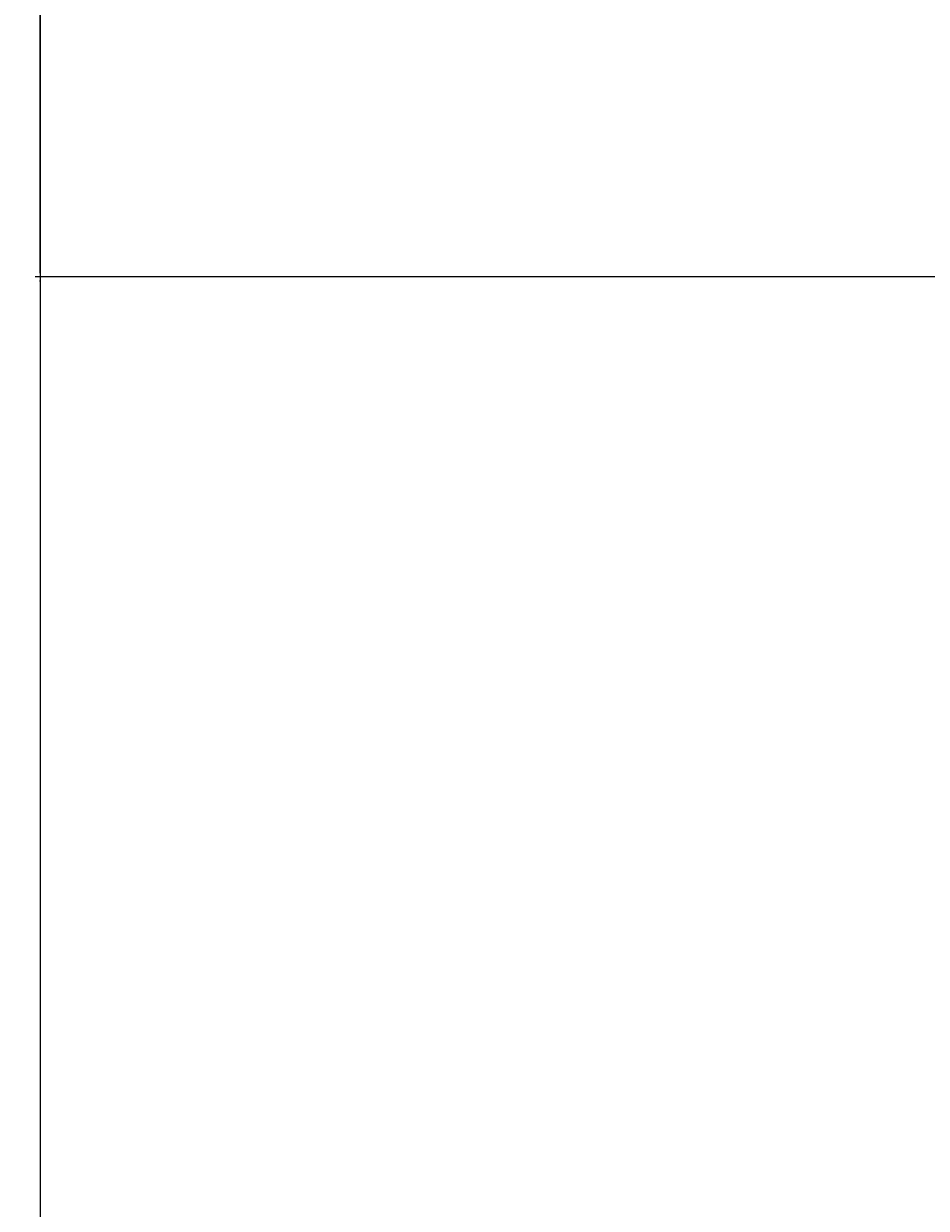
# Model space of a CAD drawing. Units: inches. Extents: x -301 to 715, y -607 to 364.
# Tile 116 of 141: x 161 to 194, y 149 to 192. Entities that reach past the tile are written whole.
import ezdxf

# ---------------------------------------------------------------- set-up
doc = ezdxf.new("R2010")
doc.units = ezdxf.units.IN
doc.header["$MEASUREMENT"] = 0
doc.layers.add('A-ANNO-DIMS', color=2, linetype='Continuous', lineweight=18)
doc.styles.get("Standard").update_dxf_attribs({"font": 'arial.ttf'})
doc.dimstyles.get("Standard").update_dxf_attribs({"dimtxt": 0.18, "dimasz": 0.18, "dimexe": 0.18, "dimexo": 0.0625, "dimgap": 0.09, "dimtad": 0, "dimtih": 1, "dimtoh": 1, "dimdec": 1, "dimzin": 0, "dimdsep": 46, "dimlunit": 4, "dimtxsty": 'Standard', "dimcen": 0.09, "dimclrd": 3, "dimclre": 4, "dimclrt": 6, "dimadec": 0, "dimazin": 0, "dimtfac": 1, "dimtdec": 1, "dimtofl": 0, "dimtmove": 0, "dimatfit": 3, "dimfxl": 1, "dimtfill": 2, "dimtfillclr": 51, "dimtolj": 1, "dimtzin": 0, "dimarcsym": 0})

# ---------------------------------------------------------------- blocks, each defined once
blk = doc.blocks.new('*D162')
at = {"layer": 'A-ANNO-DIMS', "color": 4, "lineweight": -2, "transparency": 16777216}
for p, q in [((222.328, 320.182), (161.439, 320.182)), ((222.328, -233.818), (161.439, -233.818))]:
    blk.add_line(p, q, dxfattribs=at)
at = {"layer": 'A-ANNO-DIMS', "color": 3, "lineweight": -2, "transparency": 16777216}
for p, q in [((161.619, 320.002), (161.619, 43.364)), ((161.619, -233.638), (161.619, 43))]:
    blk.add_line(p, q, dxfattribs=at)
at = {"layer": 'A-ANNO-DIMS', "color": 3, "transparency": 16777216}
for points in [[(161.589, 320.002), (161.649, 320.002), (161.619, 320.182)], [(161.589, -233.638), (161.649, -233.638), (161.619, -233.818)]]:
    blk.add_solid(points, dxfattribs=at)
at = {"layer": 'Defpoints', "color": 0, "transparency": 16777216}
for p in [(161.619, 320.182), (222.39, 320.182), (222.39, -233.818)]:
    blk.add_point(p, dxfattribs=at)
at = {"layer": 'A-ANNO-DIMS', "color": 6, "transparency": 16777216, "insert": (161.619, 43.182), "char_height": 0.18, "attachment_point": 5, "bg_fill": 1, "box_fill_scale": 1.25, "bg_fill_color": 51, "bg_fill_transparency": 0}
blk.add_mtext('\\A1;46\'-2"', dxfattribs=at)
blk = doc.blocks.new('*D169')
at = {"layer": 'A-ANNO-DIMS', "color": 4, "lineweight": -2, "transparency": 16777216}
for p, q in [((222.328, 183.182), (161.439, 183.182)), ((222.328, 55.682), (161.439, 55.682))]:
    blk.add_line(p, q, dxfattribs=at)
at = {"layer": 'A-ANNO-DIMS', "color": 3, "lineweight": -2, "transparency": 16777216}
for p, q in [((161.619, 183.002), (161.619, 119.615)), ((161.619, 55.862), (161.619, 119.249))]:
    blk.add_line(p, q, dxfattribs=at)
at = {"layer": 'A-ANNO-DIMS', "color": 3, "transparency": 16777216}
for points in [[(161.589, 183.002), (161.649, 183.002), (161.619, 183.182)], [(161.589, 55.862), (161.649, 55.862), (161.619, 55.682)]]:
    blk.add_solid(points, dxfattribs=at)
at = {"layer": 'Defpoints', "color": 0, "transparency": 16777216}
for p in [(161.619, 183.182), (222.39, 183.182), (222.39, 55.682)]:
    blk.add_point(p, dxfattribs=at)
at = {"layer": 'A-ANNO-DIMS', "color": 6, "transparency": 16777216, "insert": (161.619, 119.432), "char_height": 0.18, "attachment_point": 5, "bg_fill": 1, "box_fill_scale": 1.25, "bg_fill_color": 51, "bg_fill_transparency": 0}
blk.add_mtext('\\A1;10\'-7 1/2"', dxfattribs=at)
blk = doc.blocks.new('*D170')
at = {"layer": 'A-ANNO-DIMS', "color": 4, "lineweight": -2, "transparency": 16777216}
for p, q in [((222.328, 291.182), (161.439, 291.182)), ((222.328, 183.182), (161.439, 183.182))]:
    blk.add_line(p, q, dxfattribs=at)
at = {"layer": 'A-ANNO-DIMS', "color": 3, "lineweight": -2, "transparency": 16777216}
for p, q in [((161.619, 291.002), (161.619, 237.364)), ((161.619, 183.362), (161.619, 237))]:
    blk.add_line(p, q, dxfattribs=at)
at = {"layer": 'A-ANNO-DIMS', "color": 3, "transparency": 16777216}
for points in [[(161.589, 291.002), (161.649, 291.002), (161.619, 291.182)], [(161.589, 183.362), (161.649, 183.362), (161.619, 183.182)]]:
    blk.add_solid(points, dxfattribs=at)
at = {"layer": 'Defpoints', "color": 0, "transparency": 16777216}
for p in [(161.619, 291.182), (222.39, 291.182), (222.39, 183.182)]:
    blk.add_point(p, dxfattribs=at)
at = {"layer": 'A-ANNO-DIMS', "color": 6, "transparency": 16777216, "insert": (161.619, 237.182), "char_height": 0.18, "attachment_point": 5, "bg_fill": 1, "box_fill_scale": 1.25, "bg_fill_color": 51, "bg_fill_transparency": 0}
blk.add_mtext('\\A1;9\'-0"', dxfattribs=at)

msp = doc.modelspace()

# ---------------------------------------------------------------- dimensions: what is measured, and where the dimension line sits
at = {"layer": 'A-ANNO-DIMS'}
for base, p1, p2, picture, middle in [((161.619, 320.182), (222.39, -233.818), (222.39, 320.182), '*D162', (161.619, 43.182)), ((161.619, 291.182), (222.39, 183.182), (222.39, 291.182), '*D170', (161.619, 237.182)), ((161.619, 183.182), (222.39, 55.682), (222.39, 183.182), '*D169', (161.619, 119.432))]:
    dim = msp.add_linear_dim(base=base, p1=p1, p2=p2, angle=90, dimstyle='Standard', override={"dimdec": 1, "dimlfac": 1, "dimrnd": 0, "dimzin": 1, "dimdsep": 46, "dimlunit": 4, "dimfrac": 2}, dxfattribs=at)
    dim.commit()
    dim.dimension.update_dxf_attribs({"geometry": picture, "text_midpoint": middle})

doc.saveas('drawing.dxf')
